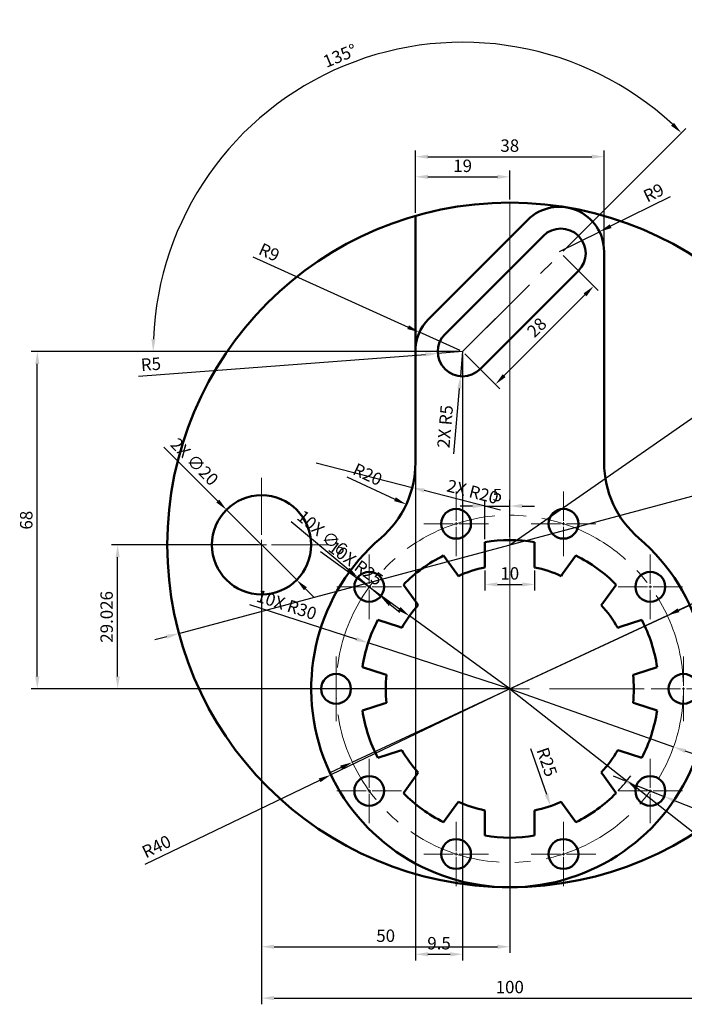
# Model space of a CAD drawing. Units: millimetres. Extents: x 3359 to 3569, y 1418 to 1617.
# Tile 1 of 2: x 3359 to 3493, y 1418 to 1617. Entities that reach past the tile are written whole.
import ezdxf

# ---------------------------------------------------------------- set-up
doc = ezdxf.new("R2010")
doc.units = ezdxf.units.MM
doc.linetypes.add('CENTER2', pattern=[28.575, 19.05, -3.175, 3.175, -3.175])
for name, color, linetype, lineweight in [('M-CNTR', 4, 'CENTER2', 18), ('M-CONS', 8, 'Continuous', 13), ('M-DIMS', 2, 'Continuous', 25), ('M-OUTL', 7, 'Continuous', 50)]:
    doc.layers.add(name, color=color, linetype=linetype, lineweight=lineweight)
doc.styles.get("Standard").update_dxf_attribs({"font": 'arial.ttf'})
doc.dimstyles.new('ISO-25', dxfattribs={"dimtxt": 2.5, "dimasz": 2.5, "dimexe": 1.25, "dimexo": 0.625, "dimtad": 1, "dimtxsty": 'Standard', "dimcen": 2.5, "dimadec": 0, "dimazin": 0, "dimtfac": 1, "dimtmove": 0, "dimatfit": 3, "dimfxl": 1, "dimarcsym": 0})

# ---------------------------------------------------------------- blocks, each defined once
blk = doc.blocks.new('*D1')
at = {"layer": 'Defpoints', "color": 0, "transparency": 16777216}
for p in [(3408.07, 1510.78), (3508.07, 1510.78), (3508.07, 1419.42)]:
    blk.add_point(p, dxfattribs=at)
at = {"layer": 'M-DIMS', "color": 0, "lineweight": -2, "transparency": 16777216}
for p, q in [((3408.07, 1510.16), (3408.07, 1418.17)), ((3508.07, 1510.16), (3508.07, 1418.17)), ((3410.57, 1419.42), (3505.57, 1419.42))]:
    blk.add_line(p, q, dxfattribs=at)
at = {"layer": 'M-DIMS', "color": 0, "transparency": 16777216}
for points in [[(3410.57, 1419.84), (3410.57, 1419), (3408.07, 1419.42)], [(3505.57, 1419.84), (3505.57, 1419), (3508.07, 1419.42)]]:
    blk.add_solid(points, dxfattribs=at)
at = {"layer": 'M-DIMS', "color": 0, "transparency": 16777216, "insert": (3458.07, 1421.32), "char_height": 2.5, "attachment_point": 5}
blk.add_mtext('100', dxfattribs=at)
blk = doc.blocks.new('*D2')
at = {"layer": 'Defpoints', "color": 0, "transparency": 16777216}
for p in [(3453.07, 1506.25), (3463.07, 1506.25), (3463.07, 1502.81)]:
    blk.add_point(p, dxfattribs=at)
at = {"layer": 'M-DIMS', "color": 0, "lineweight": -2, "transparency": 16777216}
for p, q in [((3453.07, 1505.63), (3453.07, 1501.56)), ((3463.07, 1505.63), (3463.07, 1501.56)), ((3455.57, 1502.81), (3460.57, 1502.81))]:
    blk.add_line(p, q, dxfattribs=at)
at = {"layer": 'M-DIMS', "color": 0, "transparency": 16777216}
for points in [[(3455.57, 1503.23), (3455.57, 1502.39), (3453.07, 1502.81)], [(3460.57, 1503.23), (3460.57, 1502.39), (3463.07, 1502.81)]]:
    blk.add_solid(points, dxfattribs=at)
at = {"layer": 'M-DIMS', "color": 0, "transparency": 16777216, "insert": (3458.07, 1504.71), "char_height": 2.5, "attachment_point": 5}
blk.add_mtext('10', dxfattribs=at)
blk = doc.blocks.new('*D3')
at = {"layer": 'Defpoints', "color": 0, "transparency": 16777216}
for p in [(3408.07, 1510.78), (3458.07, 1481.76), (3458.07, 1429.77)]:
    blk.add_point(p, dxfattribs=at)
at = {"layer": 'M-DIMS', "color": 0, "lineweight": -2, "transparency": 16777216}
for p, q in [((3408.07, 1510.16), (3408.07, 1428.52)), ((3458.07, 1481.13), (3458.07, 1428.52)), ((3410.57, 1429.77), (3455.57, 1429.77))]:
    blk.add_line(p, q, dxfattribs=at)
at = {"layer": 'M-DIMS', "color": 0, "transparency": 16777216}
for points in [[(3410.57, 1430.19), (3410.57, 1429.35), (3408.07, 1429.77)], [(3455.57, 1430.19), (3455.57, 1429.35), (3458.07, 1429.77)]]:
    blk.add_solid(points, dxfattribs=at)
at = {"layer": 'M-DIMS', "color": 0, "transparency": 16777216, "insert": (3433.07, 1431.67), "char_height": 2.5, "attachment_point": 5}
blk.add_mtext('50', dxfattribs=at)
blk = doc.blocks.new('*D4')
at = {"layer": 'Defpoints', "color": 0, "transparency": 16777216}
for p in [(3362.88, 1549.76), (3448.57, 1549.76), (3458.07, 1481.76)]:
    blk.add_point(p, dxfattribs=at)
at = {"layer": 'M-DIMS', "color": 0, "lineweight": -2, "transparency": 16777216}
for p, q in [((3447.94, 1549.76), (3361.63, 1549.76)), ((3362.88, 1484.26), (3362.88, 1547.26)), ((3457.44, 1481.76), (3361.63, 1481.76))]:
    blk.add_line(p, q, dxfattribs=at)
at = {"layer": 'M-DIMS', "color": 0, "transparency": 16777216}
for points in [[(3362.46, 1547.26), (3363.3, 1547.26), (3362.88, 1549.76)], [(3362.46, 1484.26), (3363.3, 1484.26), (3362.88, 1481.76)]]:
    blk.add_solid(points, dxfattribs=at)
at = {"layer": 'M-DIMS', "color": 0, "transparency": 16777216, "insert": (3360.98, 1515.76), "char_height": 2.5, "attachment_point": 5, "rotation": 90}
blk.add_mtext('68', dxfattribs=at)
blk = doc.blocks.new('*D5')
at = {"layer": 'Defpoints', "color": 0, "transparency": 16777216}
for p in [(3477.07, 1589.04), (3439.07, 1577.12), (3477.07, 1569.94)]:
    blk.add_point(p, dxfattribs=at)
at = {"layer": 'M-DIMS', "color": 0, "lineweight": -2, "transparency": 16777216}
for p, q in [((3439.07, 1577.74), (3439.07, 1590.29)), ((3477.07, 1570.57), (3477.07, 1590.29)), ((3441.57, 1589.04), (3474.57, 1589.04))]:
    blk.add_line(p, q, dxfattribs=at)
at = {"layer": 'M-DIMS', "color": 0, "transparency": 16777216}
for points in [[(3441.57, 1589.46), (3441.57, 1588.63), (3439.07, 1589.04)], [(3474.57, 1589.46), (3474.57, 1588.63), (3477.07, 1589.04)]]:
    blk.add_solid(points, dxfattribs=at)
at = {"layer": 'M-DIMS', "color": 0, "transparency": 16777216, "insert": (3458.07, 1590.95), "char_height": 2.5, "attachment_point": 5}
blk.add_mtext('38', dxfattribs=at)
blk = doc.blocks.new('*D6')
at = {"layer": 'Defpoints', "color": 0, "transparency": 16777216}
for p in [(3458.07, 1584.98), (3458.07, 1579.78), (3439.07, 1577.12)]:
    blk.add_point(p, dxfattribs=at)
at = {"layer": 'M-DIMS', "color": 0, "lineweight": -2, "transparency": 16777216}
for p, q in [((3439.07, 1577.74), (3439.07, 1586.23)), ((3458.07, 1580.41), (3458.07, 1586.23)), ((3441.57, 1584.98), (3455.57, 1584.98))]:
    blk.add_line(p, q, dxfattribs=at)
at = {"layer": 'M-DIMS', "color": 0, "transparency": 16777216}
for points in [[(3441.57, 1585.4), (3441.57, 1584.56), (3439.07, 1584.98)], [(3455.57, 1585.4), (3455.57, 1584.56), (3458.07, 1584.98)]]:
    blk.add_solid(points, dxfattribs=at)
at = {"layer": 'M-DIMS', "color": 0, "transparency": 16777216, "insert": (3448.57, 1586.88), "char_height": 2.5, "attachment_point": 5}
blk.add_mtext('19', dxfattribs=at)
blk = doc.blocks.new('*D7')
at = {"layer": 'Defpoints', "color": 0, "transparency": 16777216}
for p in [(3458.07, 1518.62), (3453.07, 1511.34), (3458.07, 1511.76)]:
    blk.add_point(p, dxfattribs=at)
at = {"layer": 'M-DIMS', "color": 0, "lineweight": -2, "transparency": 16777216}
for p, q in [((3450.57, 1518.62), (3448.07, 1518.62)), ((3453.07, 1511.96), (3453.07, 1519.87)), ((3453.07, 1518.62), (3458.07, 1518.62)), ((3458.07, 1512.38), (3458.07, 1519.87)), ((3460.57, 1518.62), (3463.07, 1518.62))]:
    blk.add_line(p, q, dxfattribs=at)
at = {"layer": 'M-DIMS', "color": 0, "transparency": 16777216}
for points in [[(3450.57, 1519.03), (3450.57, 1518.2), (3453.07, 1518.62)], [(3460.57, 1519.03), (3460.57, 1518.2), (3458.07, 1518.62)]]:
    blk.add_solid(points, dxfattribs=at)
at = {"layer": 'M-DIMS', "color": 0, "transparency": 16777216, "insert": (3455.57, 1520.51), "char_height": 2.5, "attachment_point": 5}
blk.add_mtext('5', dxfattribs=at)
blk = doc.blocks.new('*D8')
at = {"layer": 'Defpoints', "color": 0, "transparency": 16777216}
for p in [(3468.37, 1569.56), (3474.98, 1562.95), (3448.57, 1549.76)]:
    blk.add_point(p, dxfattribs=at)
at = {"layer": 'M-DIMS', "color": 0, "lineweight": -2, "transparency": 16777216}
for p, q in [((3468.81, 1569.11), (3475.86, 1562.06)), ((3456.95, 1544.91), (3473.21, 1561.18)), ((3449.01, 1549.31), (3456.06, 1542.26))]:
    blk.add_line(p, q, dxfattribs=at)
at = {"layer": 'M-DIMS', "color": 0, "transparency": 16777216}
for points in [[(3472.92, 1561.47), (3473.51, 1560.88), (3474.98, 1562.95)], [(3456.65, 1545.21), (3457.24, 1544.62), (3455.18, 1543.15)]]:
    blk.add_solid(points, dxfattribs=at)
at = {"layer": 'M-DIMS', "color": 0, "transparency": 16777216, "insert": (3463.73, 1554.39), "char_height": 2.5, "attachment_point": 5, "rotation": 45}
blk.add_mtext('28', dxfattribs=at)
blk = doc.blocks.new('*D9')
at = {"layer": 'Defpoints', "color": 0, "transparency": 16777216}
for p in [(3458.07, 1481.76), (3481.68, 1463.25)]:
    blk.add_point(p, dxfattribs=at)
at = {"layer": 'M-DIMS', "color": 0, "lineweight": -2, "transparency": 16777216}
for p, q in [((3458.07, 1481.76), (3481.68, 1463.25)), ((3516.82, 1435.71), (3483.65, 1461.71))]:
    blk.add_line(p, q, dxfattribs=at)
blk.add_arc((3458.07, 1481.76), 30, 316.7877, 324.2979, dxfattribs=at)
at = {"layer": 'M-DIMS', "color": 0, "transparency": 16777216}
blk.add_solid([(3483.91, 1462.04), (3483.39, 1461.38), (3481.68, 1463.25)], dxfattribs=at)
at = {"layer": 'M-DIMS', "color": 0, "transparency": 16777216, "insert": (3515.16, 1439.43), "char_height": 2.5, "attachment_point": 5, "rotation": 321.9105}
blk.add_mtext('R30', dxfattribs=at)
blk = doc.blocks.new('*D10')
at = {"layer": 'Defpoints', "color": 0, "transparency": 16777216}
for p in [(3458.07, 1481.76), (3491.06, 1470.06)]:
    blk.add_point(p, dxfattribs=at)
at = {"layer": 'M-DIMS', "color": 0, "lineweight": -2, "transparency": 16777216}
for p, q in [((3458.07, 1481.76), (3491.06, 1470.06)), ((3536.81, 1453.85), (3493.42, 1469.23))]:
    blk.add_line(p, q, dxfattribs=at)
at = {"layer": 'M-DIMS', "color": 0, "transparency": 16777216}
blk.add_solid([(3493.55, 1469.62), (3493.28, 1468.84), (3491.06, 1470.06)], dxfattribs=at)
at = {"layer": 'M-DIMS', "color": 0, "transparency": 16777216, "insert": (3534.03, 1456.85), "char_height": 2.5, "attachment_point": 5, "rotation": 340.485}
blk.add_mtext('R35', dxfattribs=at)
blk = doc.blocks.new('*D11')
at = {"layer": 'Defpoints', "color": 0, "transparency": 16777216}
for p in [(3458.07, 1481.76), (3422.02, 1464.42)]:
    blk.add_point(p, dxfattribs=at)
at = {"layer": 'M-DIMS', "color": 0, "lineweight": -2, "transparency": 16777216}
for p, q in [((3458.07, 1481.76), (3422.02, 1464.42)), ((3384.61, 1446.41), (3419.77, 1463.33))]:
    blk.add_line(p, q, dxfattribs=at)
at = {"layer": 'M-DIMS', "color": 0, "transparency": 16777216}
blk.add_solid([(3419.59, 1463.71), (3419.95, 1462.96), (3422.02, 1464.42)], dxfattribs=at)
at = {"layer": 'M-DIMS', "color": 0, "transparency": 16777216, "insert": (3387.03, 1449.69), "char_height": 2.5, "attachment_point": 5, "rotation": 25.6913}
blk.add_mtext('R40', dxfattribs=at)
blk = doc.blocks.new('*D12')
at = {"layer": 'Defpoints', "color": 0, "transparency": 16777216}
for p in [(3514.7, 1550.2), (3458.07, 1510.78)]:
    blk.add_point(p, dxfattribs=at)
at = {"layer": 'M-DIMS', "color": 0, "lineweight": -2, "transparency": 16777216}
for p, q in [((3524.74, 1557.19), (3516.75, 1551.63)), ((3458.07, 1510.78), (3514.7, 1550.2))]:
    blk.add_line(p, q, dxfattribs=at)
at = {"layer": 'M-DIMS', "color": 0, "transparency": 16777216}
blk.add_solid([(3516.51, 1551.97), (3516.99, 1551.29), (3514.7, 1550.2)], dxfattribs=at)
at = {"layer": 'M-DIMS', "color": 0, "transparency": 16777216, "insert": (3520.68, 1556.69), "char_height": 2.5, "attachment_point": 5, "rotation": 34.8424}
blk.add_mtext('R69', dxfattribs=at)
blk = doc.blocks.new('*D13')
at = {"layer": 'Defpoints', "color": 0, "transparency": 16777216}
for p in [(3476.14, 1573.92), (3468.07, 1569.94)]:
    blk.add_point(p, dxfattribs=at)
at = {"layer": 'M-DIMS', "color": 0, "lineweight": -2, "transparency": 16777216}
for p, q in [((3490.4, 1580.95), (3478.39, 1575.03)), ((3468.07, 1569.94), (3476.14, 1573.92))]:
    blk.add_line(p, q, dxfattribs=at)
at = {"layer": 'M-DIMS', "color": 0, "transparency": 16777216}
blk.add_solid([(3478.2, 1575.4), (3478.57, 1574.65), (3476.14, 1573.92)], dxfattribs=at)
at = {"layer": 'M-DIMS', "color": 0, "transparency": 16777216, "insert": (3487.19, 1581.49), "char_height": 2.5, "attachment_point": 5, "rotation": 26.2291}
blk.add_mtext('R9', dxfattribs=at)
blk = doc.blocks.new('*D14')
at = {"layer": 'Defpoints', "color": 0, "transparency": 16777216}
for p in [(3439.87, 1553.65), (3448.07, 1549.94)]:
    blk.add_point(p, dxfattribs=at)
at = {"layer": 'M-DIMS', "color": 0, "lineweight": -2, "transparency": 16777216}
for p, q in [((3406.28, 1568.83), (3437.59, 1554.68)), ((3448.07, 1549.94), (3439.87, 1553.65))]:
    blk.add_line(p, q, dxfattribs=at)
at = {"layer": 'M-DIMS', "color": 0, "transparency": 16777216}
blk.add_solid([(3437.76, 1555.06), (3437.42, 1554.3), (3439.87, 1553.65)], dxfattribs=at)
at = {"layer": 'M-DIMS', "color": 0, "transparency": 16777216, "insert": (3409.47, 1569.48), "char_height": 2.5, "attachment_point": 5, "rotation": 335.6781}
blk.add_mtext('R9', dxfattribs=at)
blk = doc.blocks.new('*D15')
at = {"layer": 'Defpoints', "color": 0, "transparency": 16777216}
for p in [(3443.58, 1549.38), (3448.57, 1549.76)]:
    blk.add_point(p, dxfattribs=at)
at = {"layer": 'M-DIMS', "color": 0, "lineweight": -2, "transparency": 16777216}
for p, q in [((3383.3, 1544.79), (3441.09, 1549.19)), ((3448.57, 1549.76), (3443.58, 1549.38))]:
    blk.add_line(p, q, dxfattribs=at)
at = {"layer": 'M-DIMS', "color": 0, "transparency": 16777216}
blk.add_solid([(3441.06, 1549.6), (3441.12, 1548.77), (3443.58, 1549.38)], dxfattribs=at)
at = {"layer": 'M-DIMS', "color": 0, "transparency": 16777216, "insert": (3385.79, 1546.89), "char_height": 2.5, "attachment_point": 5, "rotation": 4.3472}
blk.add_mtext('R5', dxfattribs=at)
blk = doc.blocks.new('*D16')
at = {"layer": 'Defpoints', "color": 0, "transparency": 16777216}
for p in [(3419.07, 1527.35), (3437.21, 1518.94)]:
    blk.add_point(p, dxfattribs=at)
at = {"layer": 'M-DIMS', "color": 0, "lineweight": -2, "transparency": 16777216}
blk.add_line((3425.23, 1524.5), (3434.94, 1519.99), dxfattribs=at)
at = {"layer": 'M-DIMS', "color": 0, "transparency": 16777216}
blk.add_solid([(3435.12, 1520.37), (3434.77, 1519.61), (3437.21, 1518.94)], dxfattribs=at)
at = {"layer": 'M-DIMS', "color": 0, "transparency": 16777216, "insert": (3429.3, 1524.7), "char_height": 2.5, "attachment_point": 5, "rotation": 335.1143}
blk.add_mtext('R20', dxfattribs=at)
blk = doc.blocks.new('*D17')
at = {"layer": 'Defpoints', "color": 0, "transparency": 16777216}
for p in [(3448.57, 1612.1), (3468.37, 1569.56), (3436.25, 1549.76), (3448.57, 1549.76), (3448.57, 1549.76)]:
    blk.add_point(p, dxfattribs=at)
at = {"layer": 'M-DIMS', "color": 0, "lineweight": -2, "transparency": 16777216}
for p, q in [((3468.81, 1570), (3493.54, 1594.73)), ((3435.62, 1549.76), (3384.97, 1549.76))]:
    blk.add_line(p, q, dxfattribs=at)
blk.add_arc((3448.57, 1549.76), 62.35, 47.2976, 177.7024, dxfattribs=at)
at = {"layer": 'M-DIMS', "color": 0, "transparency": 16777216}
for points in [[(3491.14, 1595.87), (3490.56, 1595.27), (3492.65, 1593.84)], [(3386.69, 1552.25), (3385.86, 1552.26), (3386.22, 1549.76)]]:
    blk.add_solid(points, dxfattribs=at)
at = {"layer": 'M-DIMS', "color": 0, "transparency": 16777216, "insert": (3423.98, 1609.11), "char_height": 2.5, "attachment_point": 5, "rotation": 22.5}
blk.add_mtext('135°', dxfattribs=at)
blk = doc.blocks.new('*D18')
at = {"layer": 'Defpoints', "color": 0, "transparency": 16777216}
for p in [(3483.6, 1462.3), (3489.17, 1460.07)]:
    blk.add_point(p, dxfattribs=at)
at = {"layer": 'M-DIMS', "color": 0, "lineweight": -2, "transparency": 16777216}
for p, q in [((3481.28, 1463.23), (3478.96, 1464.16)), ((3483.6, 1462.3), (3489.17, 1460.07)), ((3527.89, 1444.57), (3491.49, 1459.14))]:
    blk.add_line(p, q, dxfattribs=at)
at = {"layer": 'M-DIMS', "color": 0, "transparency": 16777216}
for points in [[(3481.43, 1463.61), (3481.12, 1462.84), (3483.6, 1462.3)], [(3491.65, 1459.53), (3491.34, 1458.75), (3489.17, 1460.07)]]:
    blk.add_solid(points, dxfattribs=at)
at = {"layer": 'M-DIMS', "color": 0, "transparency": 16777216, "insert": (3526.02, 1447.44), "char_height": 2.5, "attachment_point": 5, "rotation": 338.1832}
blk.add_mtext('∅6', dxfattribs=at)
blk = doc.blocks.new('*D20')
at = {"layer": 'Defpoints', "color": 0, "transparency": 16777216}
for p in [(3458.07, 1481.76), (3466.29, 1458.15)]:
    blk.add_point(p, dxfattribs=at)
at = {"layer": 'M-DIMS', "color": 0, "lineweight": -2, "transparency": 16777216}
blk.add_line((3462.26, 1469.71), (3465.47, 1460.51), dxfattribs=at)
at = {"layer": 'M-DIMS', "color": 0, "transparency": 16777216}
blk.add_solid([(3465.86, 1460.65), (3465.08, 1460.37), (3466.29, 1458.15)], dxfattribs=at)
at = {"layer": 'M-DIMS', "color": 0, "transparency": 16777216, "insert": (3465.25, 1466.91), "char_height": 2.5, "attachment_point": 5, "rotation": 289.1991}
blk.add_mtext('R25', dxfattribs=at)
blk = doc.blocks.new('*U22')
at = {"layer": 'M-CNTR', "color": 0, "transparency": 16777216}
for p, q in [((0, 2), (0, 13.5)), ((-13.5, 0), (-2, 0)), ((2, 0), (13.5, 0)), ((0, -13.5), (0, -2))]:
    blk.add_line(p, q, dxfattribs=at)
at = {"layer": 'M-CNTR', "color": 0, "linetype": 'Continuous', "transparency": 16777216}
for p, q in [((-1, 0), (1, 0)), ((0, -1), (0, 1))]:
    blk.add_line(p, q, dxfattribs=at)
blk = doc.blocks.new('*U23')
at = {"layer": 'M-CNTR', "color": 0, "transparency": 16777216}
for p, q in [((0, 8), (0, 43.5)), ((-43.5, 0), (-8, 0)), ((8, 0), (43.5, 0)), ((0, -43.5), (0, -8))]:
    blk.add_line(p, q, dxfattribs=at)
at = {"layer": 'M-CNTR', "color": 0, "linetype": 'Continuous', "transparency": 16777216}
for p, q in [((0, -4), (0, 4)), ((-4, 0), (4, 0))]:
    blk.add_line(p, q, dxfattribs=at)
blk = doc.blocks.new('*U24')
at = {"layer": 'M-CNTR', "color": 0, "transparency": 16777216}
for p, q in [((0, 0.6), (0, 6.5)), ((-6.5, 0), (-0.6, 0)), ((0.6, 0), (6.5, 0)), ((0, -6.5), (0, -0.6))]:
    blk.add_line(p, q, dxfattribs=at)
at = {"layer": 'M-CNTR', "color": 0, "linetype": 'Continuous', "transparency": 16777216}
for p, q in [((-0.3, 0), (0.3, 0)), ((0, -0.3), (0, 0.3))]:
    blk.add_line(p, q, dxfattribs=at)
blk = doc.blocks.new('*U25')
at = {"layer": 'M-CNTR', "color": 0, "transparency": 16777216}
for p, q in [((0, 0.6), (0, 6.5)), ((-6.5, 0), (-0.6, 0)), ((0.6, 0), (6.5, 0)), ((0, -6.5), (0, -0.6))]:
    blk.add_line(p, q, dxfattribs=at)
at = {"layer": 'M-CNTR', "color": 0, "linetype": 'Continuous', "transparency": 16777216}
for p, q in [((-0.3, 0), (0.3, 0)), ((0, -0.3), (0, 0.3))]:
    blk.add_line(p, q, dxfattribs=at)
blk = doc.blocks.new('*U26')
at = {"layer": 'M-CNTR', "color": 0, "transparency": 16777216}
for p, q in [((0, 0.6), (0, 6.5)), ((-6.5, 0), (-0.6, 0)), ((0.6, 0), (6.5, 0)), ((0, -6.5), (0, -0.6))]:
    blk.add_line(p, q, dxfattribs=at)
at = {"layer": 'M-CNTR', "color": 0, "linetype": 'Continuous', "transparency": 16777216}
for p, q in [((-0.3, 0), (0.3, 0)), ((0, -0.3), (0, 0.3))]:
    blk.add_line(p, q, dxfattribs=at)
blk = doc.blocks.new('*U27')
at = {"layer": 'M-CNTR', "color": 0, "transparency": 16777216}
for p, q in [((0, 0.6), (0, 6.5)), ((-6.5, 0), (-0.6, 0)), ((0.6, 0), (6.5, 0)), ((0, -6.5), (0, -0.6))]:
    blk.add_line(p, q, dxfattribs=at)
at = {"layer": 'M-CNTR', "color": 0, "linetype": 'Continuous', "transparency": 16777216}
for p, q in [((-0.3, 0), (0.3, 0)), ((0, -0.3), (0, 0.3))]:
    blk.add_line(p, q, dxfattribs=at)
blk = doc.blocks.new('*U28')
at = {"layer": 'M-CNTR', "color": 0, "transparency": 16777216}
for p, q in [((0, 0.6), (0, 6.5)), ((-6.5, 0), (-0.6, 0)), ((0.6, 0), (6.5, 0)), ((0, -6.5), (0, -0.6))]:
    blk.add_line(p, q, dxfattribs=at)
at = {"layer": 'M-CNTR', "color": 0, "linetype": 'Continuous', "transparency": 16777216}
for p, q in [((-0.3, 0), (0.3, 0)), ((0, -0.3), (0, 0.3))]:
    blk.add_line(p, q, dxfattribs=at)
blk = doc.blocks.new('*U29')
at = {"layer": 'M-CNTR', "color": 0, "transparency": 16777216}
for p, q in [((0, 0.6), (0, 6.5)), ((-6.5, 0), (-0.6, 0)), ((0.6, 0), (6.5, 0)), ((0, -6.5), (0, -0.6))]:
    blk.add_line(p, q, dxfattribs=at)
at = {"layer": 'M-CNTR', "color": 0, "linetype": 'Continuous', "transparency": 16777216}
for p, q in [((-0.3, 0), (0.3, 0)), ((0, -0.3), (0, 0.3))]:
    blk.add_line(p, q, dxfattribs=at)
blk = doc.blocks.new('*U30')
at = {"layer": 'M-CNTR', "color": 0, "transparency": 16777216}
for p, q in [((0, 0.6), (0, 6.5)), ((-6.5, 0), (-0.6, 0)), ((0.6, 0), (6.5, 0)), ((0, -6.5), (0, -0.6))]:
    blk.add_line(p, q, dxfattribs=at)
at = {"layer": 'M-CNTR', "color": 0, "linetype": 'Continuous', "transparency": 16777216}
for p, q in [((-0.3, 0), (0.3, 0)), ((0, -0.3), (0, 0.3))]:
    blk.add_line(p, q, dxfattribs=at)
blk = doc.blocks.new('*U31')
at = {"layer": 'M-CNTR', "color": 0, "transparency": 16777216}
for p, q in [((0, 0.6), (0, 6.5)), ((-6.5, 0), (-0.6, 0)), ((0.6, 0), (6.5, 0)), ((0, -6.5), (0, -0.6))]:
    blk.add_line(p, q, dxfattribs=at)
at = {"layer": 'M-CNTR', "color": 0, "linetype": 'Continuous', "transparency": 16777216}
for p, q in [((-0.3, 0), (0.3, 0)), ((0, -0.3), (0, 0.3))]:
    blk.add_line(p, q, dxfattribs=at)
blk = doc.blocks.new('*U32')
at = {"layer": 'M-CNTR', "color": 0, "transparency": 16777216}
for p, q in [((0, 0.6), (0, 6.5)), ((-6.5, 0), (-0.6, 0)), ((0.6, 0), (6.5, 0)), ((0, -6.5), (0, -0.6))]:
    blk.add_line(p, q, dxfattribs=at)
at = {"layer": 'M-CNTR', "color": 0, "linetype": 'Continuous', "transparency": 16777216}
for p, q in [((-0.3, 0), (0.3, 0)), ((0, -0.3), (0, 0.3))]:
    blk.add_line(p, q, dxfattribs=at)
blk = doc.blocks.new('*U33')
at = {"layer": 'M-CNTR', "color": 0, "transparency": 16777216}
for p, q in [((0, 0.6), (0, 6.5)), ((-6.5, 0), (-0.6, 0)), ((0.6, 0), (6.5, 0)), ((0, -6.5), (0, -0.6))]:
    blk.add_line(p, q, dxfattribs=at)
at = {"layer": 'M-CNTR', "color": 0, "linetype": 'Continuous', "transparency": 16777216}
for p, q in [((-0.3, 0), (0.3, 0)), ((0, -0.3), (0, 0.3))]:
    blk.add_line(p, q, dxfattribs=at)
blk = doc.blocks.new('BOLT-HOLE-D6')
blk.add_circle((0, 0), 3)
blk = doc.blocks.new('MOUNT-HOLE-D20')
blk.add_circle((0, 0), 10)
blk = doc.blocks.new('*D36')
at = {"layer": 'Defpoints', "color": 0, "transparency": 16777216}
for p in [(3379.07, 1510.78), (3408.07, 1510.78), (3423.07, 1481.76)]:
    blk.add_point(p, dxfattribs=at)
at = {"layer": 'M-DIMS', "color": 0, "lineweight": -2, "transparency": 16777216}
for p, q in [((3407.44, 1510.78), (3377.82, 1510.78)), ((3379.07, 1484.26), (3379.07, 1508.28)), ((3422.44, 1481.76), (3377.82, 1481.76))]:
    blk.add_line(p, q, dxfattribs=at)
at = {"layer": 'M-DIMS', "color": 0, "transparency": 16777216}
for points in [[(3378.65, 1508.28), (3379.49, 1508.28), (3379.07, 1510.78)], [(3378.65, 1484.26), (3379.49, 1484.26), (3379.07, 1481.76)]]:
    blk.add_solid(points, dxfattribs=at)
at = {"layer": 'M-DIMS', "color": 0, "transparency": 16777216, "insert": (3377.17, 1496.27), "char_height": 2.5, "attachment_point": 5, "rotation": 90}
blk.add_mtext('29.026', dxfattribs=at)
blk = doc.blocks.new('*D37')
at = {"layer": 'Defpoints', "color": 0, "transparency": 16777216}
for p in [(3448.57, 1549.76), (3439.07, 1527.35), (3448.57, 1428.26)]:
    blk.add_point(p, dxfattribs=at)
at = {"layer": 'M-DIMS', "color": 0, "lineweight": -2, "transparency": 16777216}
for p, q in [((3448.57, 1549.13), (3448.57, 1427.01)), ((3439.07, 1526.73), (3439.07, 1427.01)), ((3441.57, 1428.26), (3446.07, 1428.26))]:
    blk.add_line(p, q, dxfattribs=at)
at = {"layer": 'M-DIMS', "color": 0, "transparency": 16777216}
for points in [[(3441.57, 1428.67), (3441.57, 1427.84), (3439.07, 1428.26)], [(3446.07, 1428.67), (3446.07, 1427.84), (3448.57, 1428.26)]]:
    blk.add_solid(points, dxfattribs=at)
at = {"layer": 'M-DIMS', "color": 0, "transparency": 16777216, "insert": (3443.82, 1430.16), "char_height": 2.5, "attachment_point": 5}
blk.add_mtext('9.5', dxfattribs=at)
blk = doc.blocks.new('*D38')
at = {"layer": 'Defpoints', "color": 0, "transparency": 16777216}
for p in [(3524.72, 1528.64), (3391.42, 1492.92)]:
    blk.add_point(p, dxfattribs=at)
at = {"layer": 'M-DIMS', "color": 0, "lineweight": -2, "transparency": 16777216}
for p, q in [((3569.29, 1540.59), (3527.13, 1529.29)), ((3391.42, 1492.92), (3524.72, 1528.64)), ((3389.01, 1492.28), (3386.59, 1491.63))]:
    blk.add_line(p, q, dxfattribs=at)
at = {"layer": 'M-DIMS', "color": 0, "transparency": 16777216}
for points in [[(3527.03, 1529.69), (3527.24, 1528.89), (3524.72, 1528.64)], [(3388.9, 1492.68), (3389.11, 1491.87), (3391.42, 1492.92)]]:
    blk.add_solid(points, dxfattribs=at)
at = {"layer": 'M-DIMS', "color": 0, "transparency": 16777216, "insert": (3564.2, 1541.26), "char_height": 2.5, "attachment_point": 5, "rotation": 15.0008}
blk.add_mtext('∅138', dxfattribs=at)
blk = doc.blocks.new('*D39')
at = {"layer": 'Defpoints', "color": 0, "transparency": 16777216}
for p in [(3494.32, 1498.66), (3458.07, 1481.76)]:
    blk.add_point(p, dxfattribs=at)
at = {"layer": 'M-DIMS', "color": 0, "lineweight": -2, "transparency": 16777216}
for p, q in [((3519.34, 1510.33), (3496.59, 1499.72)), ((3458.07, 1481.76), (3494.32, 1498.66))]:
    blk.add_line(p, q, dxfattribs=at)
at = {"layer": 'M-DIMS', "color": 0, "transparency": 16777216}
blk.add_solid([(3496.41, 1500.1), (3496.76, 1499.34), (3494.32, 1498.66)], dxfattribs=at)
at = {"layer": 'M-DIMS', "color": 0, "transparency": 16777216, "insert": (3515.27, 1510.53), "char_height": 2.5, "attachment_point": 5, "rotation": 25.0008}
blk.add_mtext('R40', dxfattribs=at)
blk = doc.blocks.new('*D40')
at = {"layer": 'Defpoints', "color": 0, "transparency": 16777216}
for p in [(3489.79, 1496.55), (3426.35, 1466.96)]:
    blk.add_point(p, dxfattribs=at)
at = {"layer": 'M-DIMS', "color": 0, "lineweight": -2, "transparency": 16777216}
for p, q in [((3512.24, 1507.02), (3492.06, 1497.61)), ((3426.35, 1466.96), (3489.79, 1496.55)), ((3424.08, 1465.91), (3421.82, 1464.85))]:
    blk.add_line(p, q, dxfattribs=at)
at = {"layer": 'M-DIMS', "color": 0, "transparency": 16777216}
for points in [[(3491.88, 1497.98), (3492.23, 1497.23), (3489.79, 1496.55)], [(3423.91, 1466.29), (3424.26, 1465.53), (3426.35, 1466.96)]]:
    blk.add_solid(points, dxfattribs=at)
at = {"layer": 'M-DIMS', "color": 0, "transparency": 16777216, "insert": (3507.99, 1507.21), "char_height": 2.5, "attachment_point": 5, "rotation": 25.0014}
blk.add_mtext('∅70', dxfattribs=at)
blk = doc.blocks.new('*D41')
at = {"layer": 'Defpoints', "color": 0, "transparency": 16777216}
for p in [(3429.54, 1491.03), (3458.07, 1481.76)]:
    blk.add_point(p, dxfattribs=at)
at = {"layer": 'M-DIMS', "color": 0, "lineweight": -2, "transparency": 16777216}
for p, q in [((3405.62, 1498.8), (3427.16, 1491.8)), ((3458.07, 1481.76), (3429.54, 1491.03))]:
    blk.add_line(p, q, dxfattribs=at)
at = {"layer": 'M-DIMS', "color": 0, "transparency": 16777216}
blk.add_solid([(3427.29, 1492.2), (3427.03, 1491.4), (3429.54, 1491.03)], dxfattribs=at)
at = {"layer": 'M-DIMS', "color": 0, "transparency": 16777216, "insert": (3413.01, 1498.4), "char_height": 2.5, "attachment_point": 5, "rotation": 342.0001}
blk.add_mtext('10X R30', dxfattribs=at)
blk = doc.blocks.new('*D42')
at = {"layer": 'Defpoints', "color": 0, "transparency": 16777216}
for p in [(3437.84, 1496.45), (3458.07, 1481.76)]:
    blk.add_point(p, dxfattribs=at)
at = {"layer": 'M-DIMS', "color": 0, "lineweight": -2, "transparency": 16777216}
for p, q in [((3419.92, 1509.48), (3435.82, 1497.92)), ((3458.07, 1481.76), (3437.84, 1496.45))]:
    blk.add_line(p, q, dxfattribs=at)
at = {"layer": 'M-DIMS', "color": 0, "transparency": 16777216}
blk.add_solid([(3436.07, 1498.26), (3435.58, 1497.58), (3437.84, 1496.45)], dxfattribs=at)
at = {"layer": 'M-DIMS', "color": 0, "transparency": 16777216, "insert": (3426.83, 1506.81), "char_height": 2.5, "attachment_point": 5, "rotation": 324.0006}
blk.add_mtext('10X R25', dxfattribs=at)
blk = doc.blocks.new('*D43')
at = {"layer": 'Defpoints', "color": 0, "transparency": 16777216}
for p in [(3419.07, 1527.35), (3438.43, 1522.35)]:
    blk.add_point(p, dxfattribs=at)
at = {"layer": 'M-DIMS', "color": 0, "lineweight": -2, "transparency": 16777216}
for p, q in [((3419.07, 1527.35), (3438.43, 1522.35)), ((3456.17, 1517.77), (3440.85, 1521.72))]:
    blk.add_line(p, q, dxfattribs=at)
at = {"layer": 'M-DIMS', "color": 0, "transparency": 16777216}
blk.add_solid([(3440.96, 1522.13), (3440.75, 1521.32), (3438.43, 1522.35)], dxfattribs=at)
at = {"layer": 'M-DIMS', "color": 0, "transparency": 16777216, "insert": (3450.53, 1521.19), "char_height": 2.5, "attachment_point": 5, "rotation": 345.512}
blk.add_mtext('2X R20', dxfattribs=at)
blk = doc.blocks.new('*D44')
at = {"layer": 'Defpoints', "color": 0, "transparency": 16777216}
for p in [(3401, 1517.85), (3415.14, 1503.71)]:
    blk.add_point(p, dxfattribs=at)
at = {"layer": 'M-DIMS', "color": 0, "lineweight": -2, "transparency": 16777216}
for p, q in [((3388.4, 1530.46), (3399.23, 1519.62)), ((3415.14, 1503.71), (3401, 1517.85)), ((3416.91, 1501.94), (3418.67, 1500.17))]:
    blk.add_line(p, q, dxfattribs=at)
at = {"layer": 'M-DIMS', "color": 0, "transparency": 16777216}
for points in [[(3399.53, 1519.92), (3398.94, 1519.33), (3401, 1517.85)], [(3417.2, 1502.24), (3416.61, 1501.65), (3415.14, 1503.71)]]:
    blk.add_solid(points, dxfattribs=at)
at = {"layer": 'M-DIMS', "color": 0, "transparency": 16777216, "insert": (3394.33, 1527.32), "char_height": 2.5, "attachment_point": 5, "rotation": 314.9926}
blk.add_mtext('2X ∅20', dxfattribs=at)
blk = doc.blocks.new('*D45')
at = {"layer": 'Defpoints', "color": 0, "transparency": 16777216}
for p in [(3448.57, 1549.76), (3448.14, 1544.78)]:
    blk.add_point(p, dxfattribs=at)
at = {"layer": 'M-DIMS', "color": 0, "lineweight": -2, "transparency": 16777216}
for p, q in [((3448.57, 1549.76), (3448.14, 1544.78)), ((3446.79, 1529.12), (3447.93, 1542.28))]:
    blk.add_line(p, q, dxfattribs=at)
at = {"layer": 'M-DIMS', "color": 0, "transparency": 16777216}
blk.add_solid([(3447.51, 1542.32), (3448.34, 1542.25), (3448.14, 1544.78)], dxfattribs=at)
at = {"layer": 'M-DIMS', "color": 0, "transparency": 16777216, "insert": (3445.36, 1534.62), "char_height": 2.5, "attachment_point": 5, "rotation": 85.0704}
blk.add_mtext('2X R5', dxfattribs=at)
blk = doc.blocks.new('*D46')
at = {"layer": 'Defpoints', "color": 0, "transparency": 16777216}
for p in [(3427.45, 1504.26), (3432.05, 1500.4)]:
    blk.add_point(p, dxfattribs=at)
at = {"layer": 'M-DIMS', "color": 0, "lineweight": -2, "transparency": 16777216}
for p, q in [((3414, 1515.53), (3425.54, 1505.86)), ((3432.05, 1500.4), (3427.45, 1504.26)), ((3433.97, 1498.8), (3435.89, 1497.19))]:
    blk.add_line(p, q, dxfattribs=at)
at = {"layer": 'M-DIMS', "color": 0, "transparency": 16777216}
for points in [[(3425.81, 1506.18), (3425.27, 1505.54), (3427.45, 1504.26)], [(3434.24, 1499.12), (3433.7, 1498.48), (3432.05, 1500.4)]]:
    blk.add_solid(points, dxfattribs=at)
at = {"layer": 'M-DIMS', "color": 0, "transparency": 16777216, "insert": (3420.08, 1513.01), "char_height": 2.5, "attachment_point": 5, "rotation": 320.034}
blk.add_mtext('10X ∅6', dxfattribs=at)

msp = doc.modelspace()

# ---------------------------------------------------------------- linework, layer by layer
at = {"layer": 'M-CNTR'}
msp.add_line((3448.5696, 1549.7566), (3468.3686, 1569.5556), dxfattribs=at)
msp.add_circle((3458.0696, 1481.7566), 35, dxfattribs=at)
at = {"layer": 'M-CONS'}
for p, q in [((3458.0696, 1510.7826), (3458.0696, 1579.7826)), ((3448.5696, 1549.7566), (3458.0696, 1559.2566)), ((3435.1548, 1549.7566), (3415.9, 1549.7566)), ((3448.5696, 1549.7566), (3436.2452, 1549.7566)), ((3458.0696, 1510.7826), (3458.0696, 1544.7826)), ((3458.0696, 1544.7826), (3458.0696, 1536.7826)), ((3458.0696, 1544.7826), (3458.0696, 1476.7826)), ((3408.0696, 1510.7826), (3408.0696, 1507.2339))]:
    msp.add_line(p, q, dxfattribs=at)
at = {"layer": 'M-OUTL'}
for p, q in [((3439.0696, 1577.1151), (3439.0696, 1527.3526)), ((3461.7056, 1576.3074), (3441.7056, 1556.3074)), ((3445.034, 1553.2921), (3464.833, 1573.0911)), ((3477.0696, 1569.9434), (3477.0696, 1527.3526)), ((3452.1051, 1546.221), (3471.9041, 1566.02)), ((3439.0696, 1549.7566), (3439.0715, 1549.7566)), ((3453.0696, 1506.7566), (3453.0696, 1511.337)), ((3463.0696, 1506.7566), (3463.0696, 1511.337)), ((3447.42, 1504.9209), (3444.7277, 1508.6266)), ((3468.7191, 1504.9209), (3471.4114, 1508.6266)), ((3453.0696, 1506.7566), (3453.0696, 1506.2515)), ((3463.0696, 1506.7566), (3463.0696, 1506.2515)), ((3447.42, 1504.9209), (3447.7169, 1504.5123)), ((3468.7191, 1504.9209), (3468.4222, 1504.5123)), ((3439.3299, 1499.0431), (3436.6376, 1502.7487)), ((3476.8093, 1499.0431), (3479.5016, 1502.7487)), ((3439.3299, 1499.0431), (3439.6267, 1498.6344)), ((3476.8093, 1499.0431), (3476.5124, 1498.6344)), ((3435.8382, 1494.2373), (3431.482, 1495.6527)), ((3480.3009, 1494.2373), (3484.6571, 1495.6527)), ((3435.8382, 1494.2373), (3436.3186, 1494.0812)), ((3480.3009, 1494.2373), (3479.8205, 1494.0812)), ((3432.7481, 1484.7267), (3428.3919, 1486.1421)), ((3432.7481, 1484.7267), (3433.2285, 1484.5706)), ((3483.3911, 1484.7267), (3482.9107, 1484.5706)), ((3483.3911, 1484.7267), (3487.7473, 1486.1421)), ((3432.7481, 1478.7864), (3428.3919, 1477.371)), ((3432.7481, 1478.7864), (3433.2285, 1478.9425)), ((3483.3911, 1478.7864), (3482.9107, 1478.9425)), ((3483.3911, 1478.7864), (3487.7473, 1477.371)), ((3435.8382, 1469.2759), (3431.482, 1467.8605)), ((3435.8382, 1469.2759), (3436.3186, 1469.432)), ((3480.3009, 1469.2759), (3479.8205, 1469.432)), ((3480.3009, 1469.2759), (3484.6571, 1467.8605)), ((3439.3299, 1464.4701), (3439.6267, 1464.8787)), ((3476.8093, 1464.4701), (3476.5124, 1464.8787)), ((3439.3299, 1464.4701), (3436.6376, 1460.7645)), ((3476.8093, 1464.4701), (3479.5016, 1460.7645)), ((3447.42, 1458.5922), (3447.7169, 1459.0009)), ((3468.7191, 1458.5922), (3468.4222, 1459.0009)), ((3447.42, 1458.5922), (3444.7277, 1454.8866)), ((3453.0696, 1456.7566), (3453.0696, 1457.2617)), ((3463.0696, 1456.7566), (3463.0696, 1457.2617)), ((3468.7191, 1458.5922), (3471.4114, 1454.8866)), ((3453.0696, 1456.7566), (3453.0696, 1452.1762)), ((3463.0696, 1456.7566), (3463.0696, 1452.1762))]:
    msp.add_line(p, q, dxfattribs=at)
msp.add_circle((3458.0696, 1510.7826), 69, dxfattribs=at)
for centre, radius, start, end in [((3468.0696, 1569.9434), 9, 0, 135), ((3468.3686, 1569.5556), 5, 315, 135), ((3448.0696, 1549.9434), 9, 135, 181.189397), ((3448.5696, 1549.7566), 5, 135, 315), ((3419.0696, 1527.3526), 20, 310.541602, 0), ((3497.0696, 1527.3526), 20, 180, 229.458398), ((3458.0696, 1481.7566), 40, 130.541602, 49.458398), ((3458.0696, 1481.7566), 30, 80.405932, 99.594068), ((3458.0696, 1481.7566), 30, 116.405932, 135.594068), ((3458.0696, 1481.7566), 30, 44.405932, 63.594068), ((3458.0696, 1481.7566), 25, 101.536959, 114.463041), ((3458.0696, 1481.7566), 25, 65.536959, 78.463041), ((3458.0696, 1481.7566), 25, 137.536959, 150.463041), ((3458.0696, 1481.7566), 25, 29.536959, 42.463041), ((3458.0696, 1481.7566), 30, 152.405932, 171.594068), ((3458.0696, 1481.7566), 30, 8.405932, 27.594068), ((3458.0696, 1481.7566), 25, 173.536959, 186.463041), ((3458.0696, 1481.7566), 25, 353.536959, 6.463041), ((3458.0696, 1481.7566), 30, 188.405932, 207.594068), ((3458.0696, 1481.7566), 30, 332.405932, 351.594068), ((3458.0696, 1481.7566), 25, 209.536959, 222.463041), ((3458.0696, 1481.7566), 25, 317.536959, 330.463041), ((3458.0696, 1481.7566), 30, 224.405932, 243.594068), ((3458.0696, 1481.7566), 25, 245.536959, 258.463041), ((3458.0696, 1481.7566), 25, 281.536959, 294.463041), ((3458.0696, 1481.7566), 30, 296.405932, 315.594068), ((3458.0696, 1481.7566), 30, 260.405932, 279.594068)]:
    msp.add_arc(centre, radius, start, end, dxfattribs=at)

# ---------------------------------------------------------------- block references
at = {"layer": 'M-CNTR'}
for name, p in [('*U23', (3458.0696, 1481.7566)), ('*U22', (3408.0696, 1510.7826)), ('*U24', (3447.254, 1515.0436)), ('*U25', (3468.8852, 1515.0436)), ('*U33', (3429.754, 1502.3291)), ('*U26', (3486.3852, 1502.3291)), ('*U32', (3423.0696, 1481.7566)), ('*U27', (3493.0696, 1481.7566)), ('*U31', (3429.754, 1461.1841)), ('*U28', (3486.3852, 1461.1841)), ('*U30', (3447.254, 1448.4696)), ('*U29', (3468.8852, 1448.4696))]:
    msp.add_blockref(name, p, dxfattribs=at)
at = {"layer": 'M-OUTL'}
for name, p in [('MOUNT-HOLE-D20', (3408.0696, 1510.7826)), ('BOLT-HOLE-D6', (3447.254, 1515.0436)), ('BOLT-HOLE-D6', (3468.8852, 1515.0436)), ('BOLT-HOLE-D6', (3429.754, 1502.3291)), ('BOLT-HOLE-D6', (3486.3852, 1502.3291)), ('BOLT-HOLE-D6', (3423.0696, 1481.7566)), ('BOLT-HOLE-D6', (3493.0696, 1481.7566)), ('BOLT-HOLE-D6', (3429.754, 1461.1841)), ('BOLT-HOLE-D6', (3486.3852, 1461.1841)), ('BOLT-HOLE-D6', (3447.254, 1448.4696)), ('BOLT-HOLE-D6', (3468.8852, 1448.4696))]:
    msp.add_blockref(name, p, dxfattribs=at)

# ---------------------------------------------------------------- dimensions: what is measured, and where the dimension line sits
at = {"layer": 'M-DIMS'}
dim = msp.add_angular_dim_2l(base=(3448.5696, 1612.1025), line1=((3448.5696, 1549.7566), (3468.3686, 1569.5556)), line2=((3448.5696, 1549.7566), (3436.2452, 1549.7566)), dimstyle='ISO-25', override={"dimclrd": 0, "dimclre": 0, "dimclrt": 0}, dxfattribs=at)
dim.commit()
dim.dimension.update_dxf_attribs({"geometry": '*D17', "text_midpoint": (3423.9829, 1609.1142)})
for base, p1, p2, override, picture, middle in [((3477.0696, 1589.043), (3439.0696, 1577.1151), (3477.0696, 1569.9434), {"dimclrd": 0, "dimclre": 0, "dimclrt": 0}, '*D5', (3458.0696, 1590.9453)), ((3458.0696, 1584.981), (3439.0696, 1577.1151), (3458.0696, 1579.7826), {"dimclrd": 0, "dimclre": 0, "dimclrt": 0}, '*D6', (3448.5696, 1586.8824)), ((3448.5696, 1428.2566), (3439.0696, 1527.3526), (3448.5696, 1549.7566), {"dimdec": 1, "dimlfac": 1, "dimrnd": 0, "dimzin": 0, "dimdsep": 46, "dimlunit": 2}, '*D37', (3443.8196, 1430.158)), ((3458.0696, 1518.6182), (3453.0696, 1511.337), (3458.0696, 1511.7566), {"dimclrd": 0, "dimclre": 0, "dimclrt": 0}, '*D7', (3455.5696, 1520.5146)), ((3508.0696, 1419.4191), (3408.0696, 1510.7826), (3508.0696, 1510.7826), {"dimclrd": 0, "dimclre": 0, "dimclrt": 0}, '*D1', (3458.0696, 1421.3206)), ((3458.0696, 1429.7687), (3408.0696, 1510.7826), (3458.0696, 1481.7566), {"dimclrd": 0, "dimclre": 0, "dimclrt": 0}, '*D3', (3433.0696, 1431.6701)), ((3463.0696, 1502.8087), (3453.0696, 1506.2515), (3463.0696, 1506.2515), {"dimclrd": 0, "dimclre": 0, "dimclrt": 0}, '*D2', (3458.0696, 1504.7101))]:
    dim = msp.add_linear_dim(base=base, p1=p1, p2=p2, dimstyle='ISO-25', override=override, dxfattribs=at)
    dim.commit()
    dim.dimension.update_dxf_attribs({"geometry": picture, "text_midpoint": middle})
for center, mpoint, override, picture, middle in [((3468.0696, 1569.9434), (3476.1429, 1573.9211), {"dimclrd": 0, "dimclre": 0, "dimclrt": 0}, '*D13', (3488.0337, 1579.7796)), ((3448.0696, 1549.9434), (3439.8684, 1553.6502), {"dimclrd": 0, "dimclre": 0, "dimclrt": 0}, '*D14', (3408.6866, 1567.7436)), ((3448.5696, 1549.7566), (3443.584, 1549.3776), {"dimclrd": 0, "dimclre": 0, "dimclrt": 0}, '*D15', (3385.9384, 1544.9954)), ((3419.0696, 1527.3526), (3437.2126, 1518.9364), {"dimclrd": 0, "dimclre": 0, "dimclrt": 0}, '*D16', (3428.5007, 1522.9777)), ((3458.0696, 1481.7566), (3494.3216, 1498.6618), {"dimdec": 0, "dimlfac": 1, "dimrnd": 0, "dimzin": 0, "dimdsep": 46, "dimlunit": 2}, '*D39', (3516.0729, 1508.805)), ((3458.0696, 1481.7566), (3422.0239, 1464.4157), {"dimclrd": 0, "dimclre": 0, "dimclrt": 0}, '*D11', (3387.8565, 1447.9784)), ((3458.0696, 1481.7566), (3481.681, 1463.2498), {"dimclrd": 0, "dimclre": 0, "dimclrt": 0}, '*D9', (3513.9826, 1437.9318)), ((3458.0696, 1481.7566), (3491.059, 1470.0647), {"dimclrd": 0, "dimclre": 0, "dimclrt": 0}, '*D10', (3533.3951, 1455.0603)), ((3458.0696, 1481.7566), (3466.2909, 1458.147), {"dimclrd": 0, "dimclre": 0, "dimclrt": 0}, '*D20', (3463.4558, 1466.2888))]:
    dim = msp.add_radius_dim(center=center, mpoint=mpoint, dimstyle='ISO-25', override=override, dxfattribs=at)
    dim.commit()
    dim.dimension.update_dxf_attribs({"geometry": picture, "text_midpoint": middle, "dimtype": 164})
dim = msp.add_aligned_dim(p1=(3448.5696, 1549.7566), p2=(3468.3686, 1569.5556), distance=-9.3475, dimstyle='ISO-25', override={"dimclrd": 0, "dimclre": 0, "dimclrt": 0}, dxfattribs=at)
dim.commit()
dim.dimension.update_dxf_attribs({"geometry": '*D8', "text_midpoint": (3463.7342, 1554.3909)})
dim = msp.add_radius_dim(center=(3458.0696, 1510.7826), mpoint=(3514.6997, 1550.2038), dimstyle='ISO-25', override={"dimclrd": 0, "dimclre": 0, "dimclrt": 0}, dxfattribs=at)
dim.commit()
dim.dimension.update_dxf_attribs({"geometry": '*D12', "text_midpoint": (3520.6835, 1556.6859)})
for base, p1, p2, override, picture, middle in [((3362.8784, 1549.7566), (3458.0696, 1481.7566), (3448.5696, 1549.7566), {"dimclrd": 0, "dimclre": 0, "dimclrt": 0}, '*D4', (3360.9769, 1515.7566)), ((3379.0696, 1510.7826), (3423.0696, 1481.7566), (3408.0696, 1510.7826), {"dimdec": 3, "dimlfac": 1, "dimrnd": 0, "dimzin": 0, "dimdsep": 46, "dimlunit": 2}, '*D36', (3377.1681, 1496.2696))]:
    dim = msp.add_linear_dim(base=base, p1=p1, p2=p2, angle=90, dimstyle='ISO-25', override=override, dxfattribs=at)
    dim.commit()
    dim.dimension.update_dxf_attribs({"geometry": picture, "text_midpoint": middle})
dim = msp.add_radius_dim(center=(3448.5696, 1549.7566), mpoint=(3448.1399, 1544.7751), text='2X <>', dimstyle='ISO-25', override={"dimdec": 0, "dimlfac": 1, "dimrnd": 0, "dimzin": 0, "dimdsep": 46, "dimlunit": 2}, dxfattribs=at)
dim.commit()
dim.dimension.update_dxf_attribs({"geometry": '*D45', "text_midpoint": (3445.3555, 1534.6195)})
for p1, p2, override, picture, middle in [((3391.4209, 1492.9231), (3524.7182, 1528.6421), {"dimdec": 0, "dimlfac": 1, "dimrnd": 0, "dimzin": 0, "dimdsep": 46, "dimlunit": 2}, '*D38', (3564.7074, 1539.3577)), ((3426.3492, 1466.9642), (3489.79, 1496.549), {"dimdec": 0, "dimlfac": 1, "dimrnd": 0, "dimzin": 0, "dimdsep": 46, "dimlunit": 2}, '*D40', (3508.8222, 1505.4244)), ((3483.6, 1462.299), (3489.1703, 1460.0692), {"dimclrd": 0, "dimclre": 0, "dimclrt": 0}, '*D18', (3525.2868, 1445.6113))]:
    dim = msp.add_diameter_dim_2p(p1=p1, p2=p2, dimstyle='ISO-25', override=override, dxfattribs=at)
    dim.commit()
    dim.dimension.update_dxf_attribs({"geometry": picture, "text_midpoint": middle, "dimtype": 163})
dim = msp.add_diameter_dim_2p(p1=(3415.1397, 1503.7106), p2=(3400.9994, 1517.8546), text='2X <>', dimstyle='ISO-25', override={"dimdec": 0, "dimlfac": 1, "dimrnd": 0, "dimzin": 0, "dimdsep": 46, "dimlunit": 2}, dxfattribs=at)
dim.commit()
dim.dimension.update_dxf_attribs({"geometry": '*D44', "text_midpoint": (3392.931, 1525.9251), "dimtype": 163})
for center, mpoint, text, picture, middle in [((3419.0696, 1527.3526), (3438.4336, 1522.3491), '2X <>', '*D43', (3450.052, 1519.3469)), ((3458.0696, 1481.7566), (3437.844, 1496.451), '10X <>', '*D42', (3425.7087, 1505.2677)), ((3458.0696, 1481.7566), (3429.5379, 1491.027), '10X <>', '*D41', (3412.4188, 1496.5893))]:
    dim = msp.add_radius_dim(center=center, mpoint=mpoint, text=text, dimstyle='ISO-25', override={"dimdec": 0, "dimlfac": 1, "dimrnd": 0, "dimzin": 0, "dimdsep": 46, "dimlunit": 2}, dxfattribs=at)
    dim.commit()
    dim.dimension.update_dxf_attribs({"geometry": picture, "text_midpoint": middle, "dimtype": 164})
dim = msp.add_diameter_dim_2p(p1=(3432.0533, 1500.4021), p2=(3427.4547, 1504.2561), text='10X <>', dimstyle='ISO-25', override={"dimdec": 0, "dimlfac": 1, "dimrnd": 0, "dimzin": 0, "dimdsep": 46, "dimlunit": 2}, dxfattribs=at)
dim.commit()
dim.dimension.update_dxf_attribs({"geometry": '*D46', "text_midpoint": (3418.8121, 1511.4993)})

doc.saveas('drawing.dxf')
